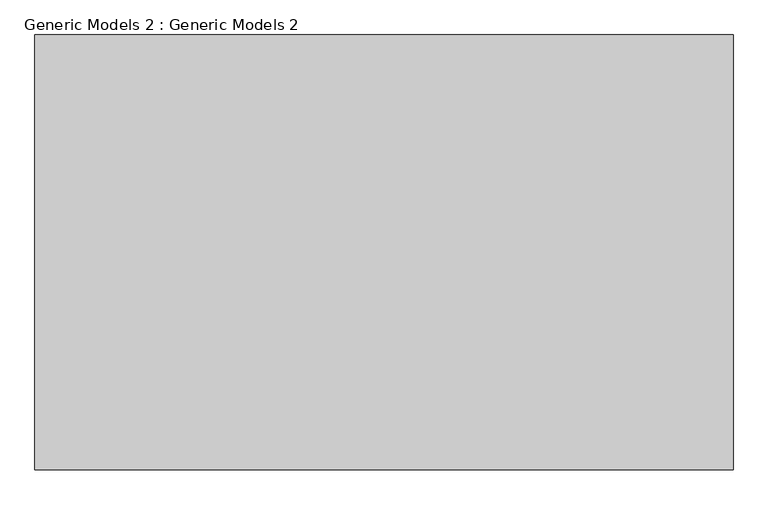
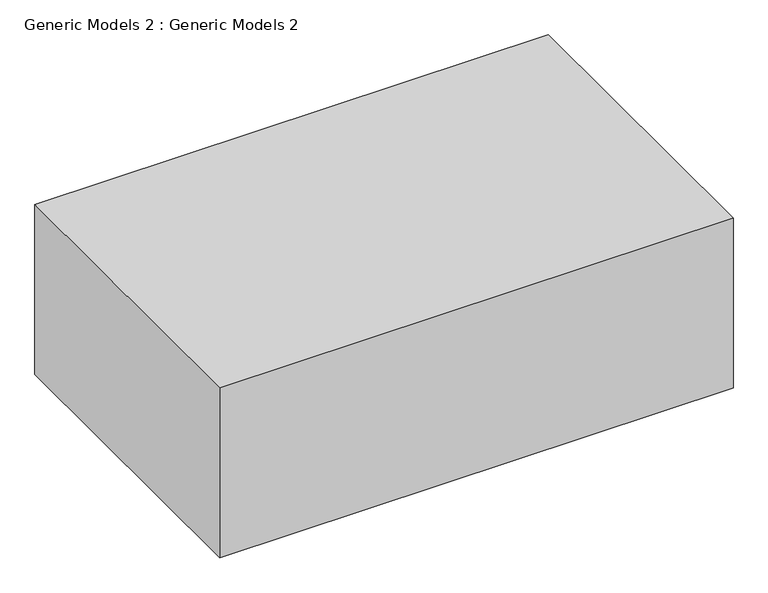
"""IFC4 building model written with IfcOpenShell, lengths in millimetres: proxy geometry, Generic Models 2 : Generic Models 2."""

from ifc_helpers import new_model, si_unit, frame, origin, place, context, project, spatial, polyline, outline, extrude, source, transform, mapped, element, save


def generic_models_2_generic_models_2_5ecfa4da(model_context):
    return source(origin(), model_context, "Body", "SweptSolid", [
        extrude(outline(polyline([(-5281.6069895, -6017.2844717), (-5281.6069895, -9246.0938957), (-10463.2069895, -9246.0938957), (-10463.2069895, -6017.2844717), (-5281.6069895, -6017.2844717)])), frame((0.0, 0.0, 6400.8), z_axis=(0.0, 0.0, 1.0), x_axis=(1.0, 0.0, 0.0)), (0.0, 0.0, 1.0), 1811.6682314),
    ])


if __name__ == "__main__":
    model = new_model("IFC4")
    model_context = context("Model", 3, world=origin())
    ifc_project = project(units=[si_unit("LENGTHUNIT", "METRE", prefix="MILLI")], contexts=[model_context])
    site = spatial("IfcSite", under=ifc_project)
    building = spatial("IfcBuilding", under=site)
    placement = place(None, origin())
    generic_models_2_generic_models_2_shape = generic_models_2_generic_models_2_5ecfa4da(model_context)
    element("IfcBuildingElementProxy", 1, Name="Generic Models 2 : Generic Models 2", ObjectType="Generic Models 2 : Generic Models 2", at=placement, inside=building, context=model_context, shape_type="MappedRepresentation", body=[
        mapped(generic_models_2_generic_models_2_shape, transform((0.0, 0.0, 0.0), x_axis=(1.0, 0.0, 0.0), y_axis=(0.0, 1.0, 0.0), z_axis=(0.0, 0.0, 1.0))),
    ])
    save(model, "model.ifc")
